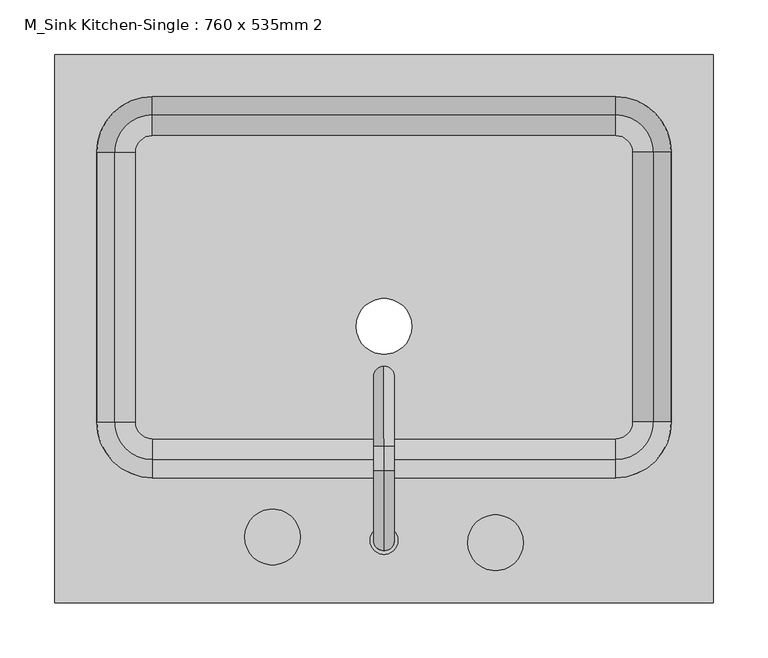
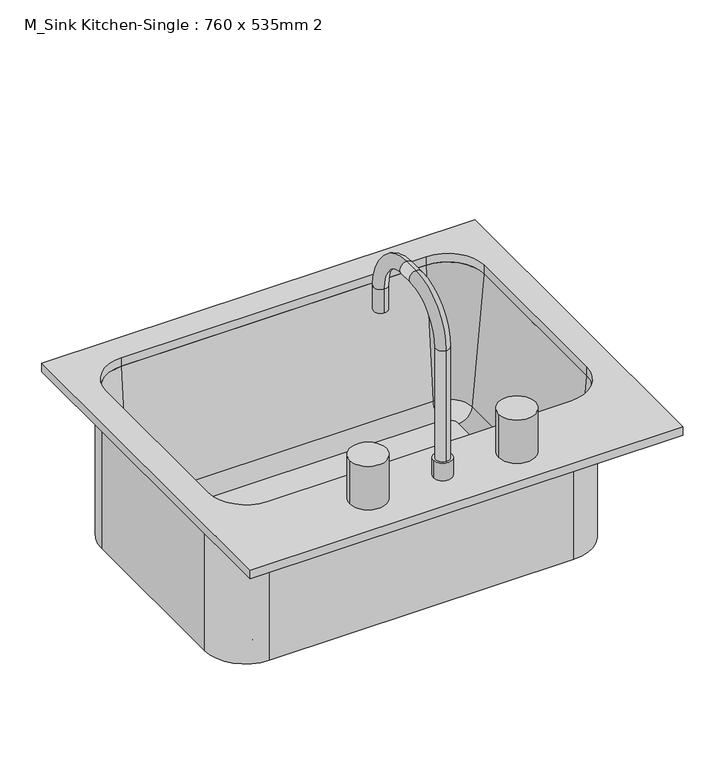
"""IFC4 building model written with IfcOpenShell, lengths in millimetres: flow terminal geometry, M_Sink Kitchen-Single : 760 x 535mm 2."""

from ifc_helpers import new_model, si_unit, point, frame, frame_2d, origin, place, context, project, spatial, polyline, circle_curve, ellipse_curve, trimmed, segment, composite_curve, outline, extrude, source, transform, mapped, element, save
from ifc_brep_helpers import plane_surface, cylinder_surface, revolved_surface, advanced_brep


def m_sink_kitchen_single_760_x_535mm_2_83ebd6f4(model_context):
    return source(origin(), model_context, "Body", "SolidModel", [
        advanced_brep(
        [(283.9392406, -87.2454011, 704.1), (283.9392406, -87.2454011, 920.0), (226.7892406, -144.3954011, 920.0), (226.7892406, -144.3954011, 704.1), (-195.4107594, -144.3954011, 704.1), (-252.5607594, -87.2454011, 704.1), (-252.5607594, 158.7545989, 704.1), (-195.4107594, 215.9045989, 704.1), (226.7892406, 215.9045989, 704.1), (283.9392406, 158.7545989, 704.1), (-9.7107594, 0.0, 704.1), (41.0892406, 0.0, 704.1), (242.0776588, -87.2454011, 713.625), (242.0776588, 158.7545989, 713.625), (226.7892406, 174.0430171, 713.625), (-195.4107594, 174.0430171, 713.625), (-210.6991776, 158.7545989, 713.625), (-210.6991776, -87.2454011, 713.625), (-195.4107594, -102.5338193, 713.625), (226.7892406, -102.5338193, 713.625), (-9.7107594, 0.0, 713.625), (41.0892406, 0.0, 713.625), (226.7892406, -121.5113283, 731.0146831), (261.0551678, -87.2454011, 731.0146831), (226.7892406, -138.0454011, 920.0), (277.5892406, -87.2454011, 920.0), (283.9392406, 158.7545989, 920.0), (261.0551678, 158.7545989, 731.0146831), (277.5892406, 158.7545989, 920.0), (226.7892406, 215.9045989, 920.0), (226.7892406, 193.0205261, 731.0146831), (226.7892406, 209.5545989, 920.0), (-195.4107594, 215.9045989, 920.0), (-195.4107594, 193.0205261, 731.0146831), (-195.4107594, 209.5545989, 920.0), (-252.5607594, 158.7545989, 920.0), (-229.6766866, 158.7545989, 731.0146831), (-246.2107594, 158.7545989, 920.0), (-252.5607594, -87.2454011, 920.0), (-229.6766866, -87.2454011, 731.0146831), (-246.2107594, -87.2454011, 920.0), (-195.4107594, -144.3954011, 920.0), (-195.4107594, -121.5113283, 731.0146831), (-195.4107594, -138.0454011, 920.0)],
        [
            (0, 1),
            (1, 2, circle_curve(frame((226.7892406, -87.2454011, 920.0), z_axis=(0.0, 0.0, -1.0), x_axis=(0.0, -1.0, 0.0)), 57.15)),
            (2, 3),
            (3, 0, circle_curve(frame((226.7892406, -87.2454011, 704.1), z_axis=(0.0, 0.0, 1.0), x_axis=(0.0, -1.0, 0.0)), 57.15)),
            (3, 4),
            (4, 5, circle_curve(frame((-195.4107594, -87.2454011, 704.1), z_axis=(0.0, 0.0, -1.0), x_axis=(-1.0, 0.0, 0.0)), 57.15)),
            (5, 6),
            (6, 7, circle_curve(frame((-195.4107594, 158.7545989, 704.1), z_axis=(0.0, 0.0, -1.0), x_axis=(0.0, 1.0, 0.0)), 57.15)),
            (7, 8),
            (8, 9, circle_curve(frame((226.7892406, 158.7545989, 704.1), z_axis=(0.0, 0.0, -1.0), x_axis=(1.0, 0.0, 0.0)), 57.15)),
            (9, 0),
            (10, 11, circle_curve(frame((15.6892406, 0.0, 704.1), z_axis=(0.0, 0.0, 1.0), x_axis=(1.0, 0.0, 0.0)), 25.4)),
            (11, 10, circle_curve(frame((15.6892406, 0.0, 704.1), z_axis=(0.0, 0.0, 1.0), x_axis=(1.0, 0.0, 0.0)), 25.4)),
            (12, 13),
            (13, 14, circle_curve(frame((226.7892406, 158.7545989, 713.625), z_axis=(0.0, 0.0, 1.0), x_axis=(1.0, 0.0, 0.0)), 15.2884182)),
            (14, 15),
            (15, 16, circle_curve(frame((-195.4107594, 158.7545989, 713.625), z_axis=(0.0, 0.0, 1.0), x_axis=(0.0, 1.0, 0.0)), 15.2884182)),
            (16, 17),
            (17, 18, circle_curve(frame((-195.4107594, -87.2454011, 713.625), z_axis=(0.0, 0.0, 1.0), x_axis=(-1.0, 0.0, 0.0)), 15.2884182)),
            (18, 19),
            (19, 12, circle_curve(frame((226.7892406, -87.2454011, 713.625), z_axis=(0.0, 0.0, 1.0), x_axis=(0.0, -1.0, 0.0)), 15.2884182)),
            (20, 21, circle_curve(frame((15.6892406, 0.0, 713.625), z_axis=(0.0, 0.0, -1.0), x_axis=(1.0, 0.0, 0.0)), 25.4)),
            (21, 20, circle_curve(frame((15.6892406, 0.0, 713.625), z_axis=(0.0, 0.0, -1.0), x_axis=(1.0, 0.0, 0.0)), 25.4)),
            (19, 22, circle_curve(frame((226.7892406, -102.5338193, 732.675), z_axis=(-1.0, 0.0, 0.0), x_axis=(0.0, -1.0, 0.0)), 19.05)),
            (22, 23, circle_curve(frame((226.7892406, -87.2454011, 731.0146831), z_axis=(0.0, 0.0, 1.0), x_axis=(0.0, -1.0, 0.0)), 34.2659272)),
            (23, 12, circle_curve(frame((242.0776588, -87.2454011, 732.675), z_axis=(0.0, 1.0, 0.0), x_axis=(1.0, 0.0, 0.0)), 19.05)),
            (22, 24),
            (24, 25, circle_curve(frame((226.7892406, -87.2454011, 920.0), z_axis=(0.0, 0.0, 1.0), x_axis=(0.0, -1.0, 0.0)), 50.8)),
            (25, 23),
            (1, 25),
            (24, 2),
            (9, 26),
            (26, 1),
            (23, 27),
            (27, 13, circle_curve(frame((242.0776588, 158.7545989, 732.675), z_axis=(0.0, 1.0, 0.0), x_axis=(1.0, 0.0, 0.0)), 19.05)),
            (25, 28),
            (28, 27),
            (26, 28),
            (8, 29),
            (29, 26, circle_curve(frame((226.7892406, 158.7545989, 920.0), z_axis=(0.0, 0.0, -1.0), x_axis=(1.0, 0.0, 0.0)), 57.15)),
            (27, 30, circle_curve(frame((226.7892406, 158.7545989, 731.0146831), z_axis=(0.0, 0.0, 1.0), x_axis=(1.0, 0.0, 0.0)), 34.2659272)),
            (30, 14, circle_curve(frame((226.7892406, 174.0430171, 732.675), z_axis=(-1.0, 0.0, 0.0), x_axis=(0.0, 1.0, 0.0)), 19.05)),
            (28, 31, circle_curve(frame((226.7892406, 158.7545989, 920.0), z_axis=(0.0, 0.0, 1.0), x_axis=(1.0, 0.0, 0.0)), 50.8)),
            (31, 30),
            (29, 31),
            (7, 32),
            (32, 29),
            (30, 33),
            (33, 15, circle_curve(frame((-195.4107594, 174.0430171, 732.675), z_axis=(-1.0, 0.0, 0.0), x_axis=(0.0, 1.0, 0.0)), 19.05)),
            (31, 34),
            (34, 33),
            (32, 34),
            (6, 35),
            (35, 32, circle_curve(frame((-195.4107594, 158.7545989, 920.0), z_axis=(0.0, 0.0, -1.0), x_axis=(0.0, 1.0, 0.0)), 57.15)),
            (33, 36, circle_curve(frame((-195.4107594, 158.7545989, 731.0146831), z_axis=(0.0, 0.0, 1.0), x_axis=(0.0, 1.0, 0.0)), 34.2659272)),
            (36, 16, circle_curve(frame((-210.6991776, 158.7545989, 732.675), z_axis=(0.0, -1.0, 0.0), x_axis=(-1.0, 0.0, 0.0)), 19.05)),
            (34, 37, circle_curve(frame((-195.4107594, 158.7545989, 920.0), z_axis=(0.0, 0.0, 1.0), x_axis=(0.0, 1.0, 0.0)), 50.8)),
            (37, 36),
            (35, 37),
            (5, 38),
            (38, 35),
            (36, 39),
            (39, 17, circle_curve(frame((-210.6991776, -87.2454011, 732.675), z_axis=(0.0, -1.0, 0.0), x_axis=(-1.0, 0.0, 0.0)), 19.05)),
            (37, 40),
            (40, 39),
            (38, 40),
            (4, 41),
            (41, 38, circle_curve(frame((-195.4107594, -87.2454011, 920.0), z_axis=(0.0, 0.0, -1.0), x_axis=(-1.0, 0.0, 0.0)), 57.15)),
            (39, 42, circle_curve(frame((-195.4107594, -87.2454011, 731.0146831), z_axis=(0.0, 0.0, 1.0), x_axis=(-1.0, 0.0, 0.0)), 34.2659272)),
            (42, 18, circle_curve(frame((-195.4107594, -102.5338193, 732.675), z_axis=(1.0, 0.0, 0.0), x_axis=(0.0, -1.0, 0.0)), 19.05)),
            (40, 43, circle_curve(frame((-195.4107594, -87.2454011, 920.0), z_axis=(0.0, 0.0, 1.0), x_axis=(-1.0, 0.0, 0.0)), 50.8)),
            (43, 42),
            (41, 43),
            (2, 41),
            (42, 22),
            (43, 24),
            (21, 11),
            (10, 20),
        ],
        [
            cylinder_surface(frame((226.7892406, -87.2454011, 0.0), z_axis=(0.0, 0.0, -1.0), x_axis=(0.0, -1.0, 0.0)), 57.15),
            plane_surface(frame((226.7892406, -87.2454011, 704.1), z_axis=(0.0, 0.0, -1.0), x_axis=(0.0, -1.0, 0.0))),
            plane_surface(frame((226.7892406, -87.2454011, 713.625), z_axis=(0.0, 0.0, 1.0), x_axis=(0.0, -1.0, 0.0))),
            revolved_surface(trimmed(ellipse_curve(frame((226.7892406, -102.5338193, 732.675), z_axis=(-1.0, 0.0, 0.0), x_axis=(0.0, -1.0, 0.0)), 19.05, 19.05), [point((226.7892406, -102.5338193, 713.625))], [point((226.7892406, -121.5113283, 731.0146831))], True, "CARTESIAN"), (226.7892406, -87.2454011, 0.0), (0.0, 0.0, -1.0)),
            revolved_surface(polyline([(226.7892406, -121.5113283, 731.0146831), (226.7892406, -138.0454011, 920.0)]), (226.7892406, -87.2454011, 0.0), (0.0, 0.0, -1.0)),
            plane_surface(frame((226.7892406, -87.2454011, 920.0), z_axis=(0.0, 0.0, 1.0), x_axis=(0.0, -1.0, 0.0))),
            plane_surface(frame((283.9392406, -87.2454011, 920.0), z_axis=(1.0, 0.0, 0.0), x_axis=(0.0, 1.0, 0.0))),
            revolved_surface(polyline([(261.1276588, 158.75459890000002, 732.675), (261.1276588, -87.2454011, 732.675)]), (242.0776588, -87.2454011, 732.675), (0.0, 1.0, 0.0)),
            plane_surface(frame((261.0551678, -87.2454011, 731.0146831), z_axis=(-0.9961946980917443, 0.0, 0.08715574274767207), x_axis=(0.0, 1.0, 0.0))),
            plane_surface(frame((277.5892406, -87.2454011, 920.0), z_axis=(0.0, 0.0, 1.0), x_axis=(0.0, 1.0, 0.0))),
            cylinder_surface(frame((226.7892406, 158.7545989, 0.0), z_axis=(0.0, 0.0, -1.0), x_axis=(1.0, 0.0, 0.0)), 57.15),
            revolved_surface(trimmed(ellipse_curve(frame((242.0776588, 158.7545989, 732.675), z_axis=(0.0, -1.0, 0.0), x_axis=(1.0, 0.0, 0.0)), 19.05, 19.05), [point((242.0776588, 158.7545989, 713.625))], [point((261.0551678, 158.7545989, 731.0146831))], True, "CARTESIAN"), (226.7892406, 158.7545989, 0.0), (0.0, 0.0, -1.0)),
            revolved_surface(polyline([(261.0551678, 158.7545989, 731.0146831), (277.5892406, 158.7545989, 920.0)]), (226.7892406, 158.7545989, 0.0), (0.0, 0.0, -1.0)),
            plane_surface(frame((226.7892406, 158.7545989, 920.0), z_axis=(0.0, 0.0, 1.0), x_axis=(1.0, 0.0, 0.0))),
            plane_surface(frame((226.7892406, 215.9045989, 920.0), z_axis=(0.0, 1.0, 0.0), x_axis=(-1.0, 0.0, 0.0))),
            revolved_surface(polyline([(-195.4107594, 193.0930171, 732.675), (226.7892406, 193.0930171, 732.675)]), (226.7892406, 174.0430171, 732.675), (-1.0, 0.0, 0.0)),
            plane_surface(frame((226.7892406, 193.0205261, 731.0146831), z_axis=(0.0, -0.9961946980917443, 0.08715574274767207), x_axis=(-1.0, 0.0, 0.0))),
            plane_surface(frame((226.7892406, 209.5545989, 920.0), z_axis=(0.0, 0.0, 1.0), x_axis=(-1.0, 0.0, 0.0))),
            cylinder_surface(frame((-195.4107594, 158.7545989, 0.0), z_axis=(0.0, 0.0, -1.0), x_axis=(0.0, 1.0, 0.0)), 57.15),
            revolved_surface(trimmed(ellipse_curve(frame((-195.4107594, 174.0430171, 732.675), z_axis=(1.0, 0.0, 0.0), x_axis=(0.0, 1.0, 0.0)), 19.05, 19.05), [point((-195.4107594, 174.0430171, 713.625))], [point((-195.4107594, 193.0205261, 731.0146831))], True, "CARTESIAN"), (-195.4107594, 158.7545989, 0.0), (0.0, 0.0, -1.0)),
            revolved_surface(polyline([(-195.4107594, 193.0205261, 731.0146831), (-195.4107594, 209.5545989, 920.0)]), (-195.4107594, 158.7545989, 0.0), (0.0, 0.0, -1.0)),
            plane_surface(frame((-195.4107594, 158.7545989, 920.0), z_axis=(0.0, 0.0, 1.0), x_axis=(0.0, 1.0, 0.0))),
            plane_surface(frame((-252.5607594, 158.7545989, 920.0), z_axis=(-1.0, 0.0, 0.0), x_axis=(0.0, -1.0, 0.0))),
            revolved_surface(polyline([(-229.74917760000002, -87.24540110000001, 732.675), (-229.74917760000002, 158.7545989, 732.675)]), (-210.6991776, 158.7545989, 732.675), (0.0, -1.0, 0.0)),
            plane_surface(frame((-229.6766866, 158.7545989, 731.0146831), z_axis=(0.9961946980917443, 0.0, 0.08715574274767207), x_axis=(0.0, -1.0, 0.0))),
            plane_surface(frame((-246.2107594, 158.7545989, 920.0), z_axis=(0.0, 0.0, 1.0), x_axis=(0.0, -1.0, 0.0))),
            cylinder_surface(frame((-195.4107594, -87.2454011, 0.0), z_axis=(0.0, 0.0, -1.0), x_axis=(-1.0, 0.0, 0.0)), 57.15),
            revolved_surface(trimmed(ellipse_curve(frame((-210.6991776, -87.2454011, 732.675), z_axis=(0.0, 1.0, 0.0), x_axis=(-1.0, 0.0, 0.0)), 19.05, 19.05), [point((-210.6991776, -87.2454011, 713.625))], [point((-229.6766866, -87.2454011, 731.0146831))], True, "CARTESIAN"), (-195.4107594, -87.2454011, 0.0), (0.0, 0.0, -1.0)),
            revolved_surface(polyline([(-229.6766866, -87.2454011, 731.0146831), (-246.2107594, -87.2454011, 920.0)]), (-195.4107594, -87.2454011, 0.0), (0.0, 0.0, -1.0)),
            plane_surface(frame((-195.4107594, -87.2454011, 920.0), z_axis=(0.0, 0.0, 1.0), x_axis=(-1.0, 0.0, 0.0))),
            plane_surface(frame((-195.4107594, -144.3954011, 920.0), z_axis=(0.0, -1.0, 0.0), x_axis=(1.0, 0.0, 0.0))),
            revolved_surface(polyline([(226.7892406, -121.5838193, 732.675), (-195.4107594, -121.5838193, 732.675)]), (-195.4107594, -102.5338193, 732.675), (1.0, 0.0, 0.0)),
            plane_surface(frame((-195.4107594, -121.5113283, 731.0146831), z_axis=(0.0, 0.9961946980917443, 0.08715574274767207), x_axis=(1.0, 0.0, 0.0))),
            plane_surface(frame((-195.4107594, -138.0454011, 920.0), z_axis=(0.0, 0.0, 1.0), x_axis=(1.0, 0.0, 0.0))),
            revolved_surface(polyline([(41.0892406, 0.0, 704.1), (41.0892406, 0.0, 713.625)]), (15.6892406, 0.0, 0.0), (0.0, 0.0, -1.0)),
        ],
        [
            (0, [[1, 2, 3, 4]]),
            (1, [[5, 6, 7, 8, 9, 10, 11, -4], [12, 13]]),
            (2, [[14, 15, 16, 17, 18, 19, 20, 21], [22, 23]]),
            (3, [[24, 25, 26, -21]]),
            (4, [[27, 28, 29, -25]]),
            (5, [[30, -28, 31, -2]]),
            (6, [[-11, 32, 33, -1]]),
            (7, [[34, 35, -14, -26]]),
            (8, [[36, 37, -34, -29]]),
            (9, [[-33, 38, -36, -30]]),
            (10, [[-10, 39, 40, -32]]),
            (11, [[41, 42, -15, -35]]),
            (12, [[43, 44, -41, -37]]),
            (13, [[-40, 45, -43, -38]]),
            (14, [[-9, 46, 47, -39]]),
            (15, [[48, 49, -16, -42]]),
            (16, [[50, 51, -48, -44]]),
            (17, [[-47, 52, -50, -45]]),
            (18, [[-8, 53, 54, -46]]),
            (19, [[55, 56, -17, -49]]),
            (20, [[57, 58, -55, -51]]),
            (21, [[-54, 59, -57, -52]]),
            (22, [[-7, 60, 61, -53]]),
            (23, [[62, 63, -18, -56]]),
            (24, [[64, 65, -62, -58]]),
            (25, [[-61, 66, -64, -59]]),
            (26, [[-6, 67, 68, -60]]),
            (27, [[69, 70, -19, -63]]),
            (28, [[71, 72, -69, -65]]),
            (29, [[-68, 73, -71, -66]]),
            (30, [[74, -67, -5, -3]]),
            (31, [[-20, -70, 75, -24]]),
            (32, [[-75, -72, 76, -27]]),
            (33, [[-76, -73, -74, -31]]),
            (34, [[77, -12, 78, -23]]),
            (34, [[-78, -13, -77, -22]]),
        ],
    ),
        advanced_brep(
        [(2.9892406, -195.1954011, 958.1), (28.3892406, -195.1954011, 958.1), (15.6892406, -204.7204011, 958.1), (15.6892406, -185.6704011, 958.1), (2.9892406, -195.1954011, 932.7), (28.3892406, -195.1954011, 932.7), (15.6892406, -204.7204011, 1120.025), (15.6892406, -185.6704011, 1120.025), (15.6892406, -131.6954011, 1174.0), (15.6892406, -131.6954011, 1193.05), (15.6892406, -109.4704011, 1174.0), (15.6892406, -109.4704011, 1193.05), (15.6892406, -55.4954011, 1120.025), (15.6892406, -36.4454011, 1120.025), (15.6892406, -36.4454011, 1085.1), (15.6892406, -55.4954011, 1085.1)],
        [
            (0, 1, circle_curve(frame((15.6892406, -195.1954011, 958.1), z_axis=(0.0, 0.0, 1.0), x_axis=(1.0, 0.0, 0.0)), 12.7)),
            (1, 0, circle_curve(frame((15.6892406, -195.1954011, 958.1), z_axis=(0.0, 0.0, 1.0), x_axis=(1.0, 0.0, 0.0)), 12.7)),
            (2, 3, circle_curve(frame((15.6892406, -195.1954011, 958.1), z_axis=(0.0, 0.0, -1.0), x_axis=(0.0, 1.0, 0.0)), 9.525)),
            (3, 2, circle_curve(frame((15.6892406, -195.1954011, 958.1), z_axis=(0.0, 0.0, -1.0), x_axis=(0.0, 1.0, 0.0)), 9.525)),
            (4, 5, circle_curve(frame((15.6892406, -195.1954011, 932.7), z_axis=(0.0, 0.0, -1.0), x_axis=(1.0, 0.0, 0.0)), 12.7)),
            (5, 4, circle_curve(frame((15.6892406, -195.1954011, 932.7), z_axis=(0.0, 0.0, -1.0), x_axis=(1.0, 0.0, 0.0)), 12.7)),
            (1, 5),
            (4, 0),
            (6, 2),
            (3, 7),
            (7, 6, circle_curve(frame((15.6892406, -195.1954011, 1120.025), z_axis=(0.0, 0.0, -1.0), x_axis=(0.0, 1.0, 0.0)), 9.525)),
            (6, 7, circle_curve(frame((15.6892406, -195.1954011, 1120.025), z_axis=(0.0, 0.0, -1.0), x_axis=(0.0, 1.0, 0.0)), 9.525)),
            (7, 8, circle_curve(frame((15.6892406, -131.6954011, 1120.025), z_axis=(-1.0, 0.0, 0.0), x_axis=(0.0, -1.0, 0.0)), 53.975)),
            (8, 9, circle_curve(frame((15.6892406, -131.6954011, 1183.525), z_axis=(0.0, -1.0, 0.0), x_axis=(0.0, 0.0, -1.0)), 9.525)),
            (9, 6, circle_curve(frame((15.6892406, -131.6954011, 1120.025), z_axis=(1.0, 0.0, 0.0), x_axis=(0.0, -1.0, 0.0)), 73.025)),
            (9, 8, circle_curve(frame((15.6892406, -131.6954011, 1183.525), z_axis=(0.0, -1.0, 0.0), x_axis=(0.0, 0.0, -1.0)), 9.525)),
            (8, 10),
            (10, 11, circle_curve(frame((15.6892406, -109.4704011, 1183.525), z_axis=(0.0, -1.0, 0.0), x_axis=(0.0, 0.0, -1.0)), 9.525)),
            (11, 9),
            (11, 10, circle_curve(frame((15.6892406, -109.4704011, 1183.525), z_axis=(0.0, -1.0, 0.0), x_axis=(0.0, 0.0, -1.0)), 9.525)),
            (10, 12, circle_curve(frame((15.6892406, -109.4704011, 1120.025), z_axis=(-1.0, 0.0, 0.0), x_axis=(0.0, 0.0, 1.0)), 53.975)),
            (12, 13, circle_curve(frame((15.6892406, -45.9704011, 1120.025), z_axis=(0.0, 0.0, 1.0), x_axis=(0.0, -1.0, 0.0)), 9.525)),
            (13, 11, circle_curve(frame((15.6892406, -109.4704011, 1120.025), z_axis=(1.0, 0.0, 0.0), x_axis=(0.0, 0.0, 1.0)), 73.025)),
            (13, 12, circle_curve(frame((15.6892406, -45.9704011, 1120.025), z_axis=(0.0, 0.0, 1.0), x_axis=(0.0, -1.0, 0.0)), 9.525)),
            (14, 15, circle_curve(frame((15.6892406, -45.9704011, 1085.1), z_axis=(0.0, 0.0, -1.0), x_axis=(0.0, -1.0, 0.0)), 9.525)),
            (15, 14, circle_curve(frame((15.6892406, -45.9704011, 1085.1), z_axis=(0.0, 0.0, -1.0), x_axis=(0.0, -1.0, 0.0)), 9.525)),
            (12, 15),
            (14, 13),
        ],
        [
            plane_surface(frame((28.3892406, -195.1954011, 958.1), z_axis=(0.0, 0.0, 1.0), x_axis=(0.0, -1.0, 0.0))),
            plane_surface(frame((28.3892406, -195.1954011, 932.7), z_axis=(0.0, 0.0, -1.0), x_axis=(0.0, 1.0, 0.0))),
            cylinder_surface(frame((15.6892406, -195.1954011, 932.7), z_axis=(0.0, 0.0, 1.0), x_axis=(1.0, 0.0, 0.0)), 12.7),
            cylinder_surface(frame((15.6892406, -195.1954011, 932.7), z_axis=(0.0, 0.0, -1.0), x_axis=(0.0, 1.0, 0.0)), 9.525),
            revolved_surface(trimmed(ellipse_curve(frame((15.6892406, -195.1954011, 1120.025), z_axis=(0.0, 0.0, 1.0), x_axis=(0.0, 1.0, 0.0)), 9.525, 9.525), [point((15.6892406, -204.7204011, 1120.025))], [point((15.6892406, -185.6704011, 1120.025))], True, "CARTESIAN"), (15.6892406, -131.6954011, 1120.025), (1.0, 0.0, 0.0)),
            revolved_surface(trimmed(ellipse_curve(frame((15.6892406, -195.1954011, 1120.025), z_axis=(0.0, 0.0, 1.0), x_axis=(0.0, 1.0, 0.0)), 9.525, 9.525), [point((15.6892406, -185.6704011, 1120.025))], [point((15.6892406, -204.7204011, 1120.025))], True, "CARTESIAN"), (15.6892406, -131.6954011, 1120.025), (1.0, 0.0, 0.0)),
            cylinder_surface(frame((15.6892406, -131.6954011, 1183.525), z_axis=(0.0, -1.0, 0.0), x_axis=(0.0, 0.0, -1.0)), 9.525),
            revolved_surface(trimmed(ellipse_curve(frame((15.6892406, -109.4704011, 1183.525), z_axis=(0.0, 1.0, 0.0), x_axis=(0.0, 0.0, -1.0)), 9.525, 9.525), [point((15.6892406, -109.4704011, 1193.05))], [point((15.6892406, -109.4704011, 1174.0))], True, "CARTESIAN"), (15.6892406, -109.4704011, 1120.025), (1.0, 0.0, 0.0)),
            revolved_surface(trimmed(ellipse_curve(frame((15.6892406, -109.4704011, 1183.525), z_axis=(0.0, 1.0, 0.0), x_axis=(0.0, 0.0, -1.0)), 9.525, 9.525), [point((15.6892406, -109.4704011, 1174.0))], [point((15.6892406, -109.4704011, 1193.05))], True, "CARTESIAN"), (15.6892406, -109.4704011, 1120.025), (1.0, 0.0, 0.0)),
            plane_surface(frame((15.6892406, -36.4454011, 1085.1), z_axis=(0.0, 0.0, -1.0), x_axis=(-1.0, 0.0, 0.0))),
            cylinder_surface(frame((15.6892406, -45.9704011, 1120.025), z_axis=(0.0, 0.0, 1.0), x_axis=(0.0, -1.0, 0.0)), 9.525),
        ],
        [
            (0, [[1, 2], [3, 4]]),
            (1, [[5, 6]]),
            (2, [[7, -5, 8, -2]]),
            (2, [[-8, -6, -7, -1]]),
            (3, [[9, -4, 10, 11]]),
            (3, [[-10, -3, -9, 12]]),
            (4, [[13, 14, 15, -11]]),
            (5, [[-15, 16, -13, -12]]),
            (6, [[17, 18, 19, -14]]),
            (6, [[-19, 20, -17, -16]]),
            (7, [[21, 22, 23, -18]]),
            (8, [[-23, 24, -21, -20]]),
            (9, [[25, 26]]),
            (10, [[27, -25, 28, -22]]),
            (10, [[-28, -26, -27, -24]]),
        ],
    ),
        extrude(outline(composite_curve([segment(trimmed(circle_curve(frame_2d((-85.9107594, -192.1166076)), 25.4), [point((-111.3107594, -192.1166076))], [point((-60.5107594, -192.1166076))], False, "CARTESIAN"), True, "CONTINUOUS"), segment(trimmed(circle_curve(frame_2d((-85.9107594, -192.1166076)), 25.4), [point((-60.5107594, -192.1166076))], [point((-111.3107594, -192.1166076))], False, "CARTESIAN"), True, "CONTINUOUS")], self_intersect=False)), frame((0.0, 0.0, 932.7), z_axis=(0.0, 0.0, 1.0), x_axis=(1.0, 0.0, 0.0)), (0.0, 0.0, 1.0), 63.5),
        extrude(outline(composite_curve([segment(trimmed(circle_curve(frame_2d((117.2892406, -197.3133323)), 25.4), [point((91.8892406, -197.3133323))], [point((142.6892406, -197.3133323))], False, "CARTESIAN"), True, "CONTINUOUS"), segment(trimmed(circle_curve(frame_2d((117.2892406, -197.3133323)), 25.4), [point((142.6892406, -197.3133323))], [point((91.8892406, -197.3133323))], False, "CARTESIAN"), True, "CONTINUOUS")], self_intersect=False)), frame((0.0, 0.0, 932.7), z_axis=(0.0, 0.0, 1.0), x_axis=(1.0, 0.0, 0.0)), (0.0, 0.0, 1.0), 63.5),
        extrude(outline(polyline([(315.6892406, -252.3454011), (-284.3107594, -252.3454011), (-284.3107594, 247.6545989), (315.6892406, 247.6545989), (315.6892406, -252.3454011)]), holes=[composite_curve([segment(trimmed(circle_curve(frame_2d((226.7892406, -87.2454011)), 50.8), [point((226.7892406, -138.0454011))], [point((277.5892406, -87.2454011))], True, "CARTESIAN"), True, "CONTINUOUS"), segment(polyline([(277.5892406, -87.2454011), (277.5892406, 158.7545989)]), True, "CONTINUOUS"), segment(trimmed(circle_curve(frame_2d((226.7892406, 158.7545989)), 50.8), [point((277.5892406, 158.7545989))], [point((226.7892406, 209.5545989))], True, "CARTESIAN"), True, "CONTINUOUS"), segment(polyline([(226.7892406, 209.5545989), (-195.4107594, 209.5545989)]), True, "CONTINUOUS"), segment(trimmed(circle_curve(frame_2d((-195.4107594, 158.7545989)), 50.8), [point((-195.4107594, 209.5545989))], [point((-246.2107594, 158.7545989))], True, "CARTESIAN"), True, "CONTINUOUS"), segment(polyline([(-246.2107594, 158.7545989), (-246.2107594, -87.2454011)]), True, "CONTINUOUS"), segment(trimmed(circle_curve(frame_2d((-195.4107594, -87.2454011)), 50.8), [point((-246.2107594, -87.2454011))], [point((-195.4107594, -138.0454011))], True, "CARTESIAN"), True, "CONTINUOUS"), segment(polyline([(-195.4107594, -138.0454011), (226.7892406, -138.0454011)]), True, "CONTINUOUS")], self_intersect=False)]), frame((0.0, 0.0, 920.0), z_axis=(0.0, 0.0, 1.0), x_axis=(1.0, 0.0, 0.0)), (0.0, 0.0, 1.0), 12.7),
    ])


if __name__ == "__main__":
    model = new_model("IFC4")
    model_context = context("Model", 3, world=origin())
    ifc_project = project(units=[si_unit("LENGTHUNIT", "METRE", prefix="MILLI")], contexts=[model_context])
    site = spatial("IfcSite", under=ifc_project)
    building = spatial("IfcBuilding", under=site)
    placement = place(None, origin())
    m_sink_kitchen_single_760_x_535mm_2_shape = m_sink_kitchen_single_760_x_535mm_2_83ebd6f4(model_context)
    element("IfcFlowTerminal", 1, ObjectType="M_Sink Kitchen-Single : 760 x 535mm 2", at=placement, inside=building, context=model_context, shape_type="MappedRepresentation", body=[
        mapped(m_sink_kitchen_single_760_x_535mm_2_shape, transform((0.0, 0.0, 0.0), x_axis=(1.0, 0.0, 0.0), y_axis=(0.0, 1.0, 0.0), z_axis=(0.0, 0.0, 1.0))),
    ])
    save(model, "model.ifc")

# Revit data of these elements
# Type "M_Sink Kitchen-Single : 760 x 535mm 2"
#   Counter Height = 3' - 0.22047"
#   Depth = 1' - 7.68504"
#   Width = 1' - 11.62205"
#   Fixture Material = Metal - Steel, Polished
#   Sink Material = Metal - Steel, Polished
#   Default Elevation = 0
#   Assembly Code = ""
# Element 1 (IfcFlowTerminal, "M_Sink Kitchen-Single : 760 x 535mm 2")
#   Materials on its faces: "Metal - Steel, Polished"
# Materials
#   "Metal - Steel, Polished": class "Metal", colour RGB 192 192 192, transparency 0
